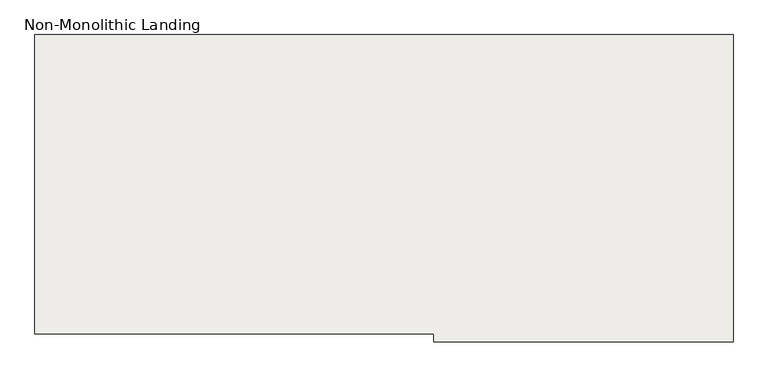
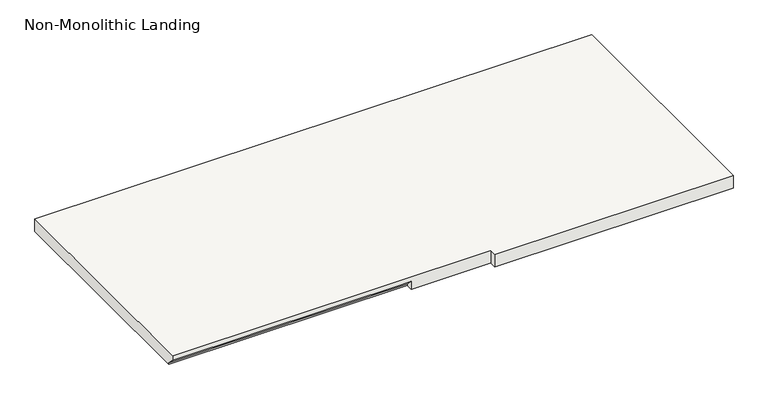
"""IFC4 building model written with IfcOpenShell, lengths in millimetres: slab geometry, Non-Monolithic Landing."""

from ifc_helpers import new_model, si_unit, origin, place, context, project, spatial, faceted_brep, source, transform, mapped, element, save


def non_monolithic_landing_da8bd63b(model_context):
    return source(origin(), model_context, "Body", "Brep", [
        faceted_brep([(-3617.4415084, 23194.7216096, 48752.9005799), (-3617.4415084, 23220.1216096, 48727.5005799), (-2703.0415084, 23220.1216096, 48727.5005799), (-2703.0415084, 23194.7216096, 48752.9005799), (-2398.2415084, 23194.7216096, 48771.9505799), (-2398.2415084, 23169.3216096, 48771.9505799), (-1483.8415084, 23169.3216096, 48771.9505799), (-1483.8415084, 23194.7216096, 48771.9505799), (-1483.8415084, 24109.1216096, 48771.9505799), (-3617.4415084, 24109.1216096, 48771.9505799), (-3617.4415084, 23194.7216096, 48771.9505799), (-2703.0415084, 23220.1216096, 48721.1505799), (-3617.4415084, 23220.1216096, 48721.1505799), (-3617.4415084, 24109.1216096, 48721.1505799), (-1483.8415084, 24109.1216096, 48721.1505799), (-1483.8415084, 23194.7216096, 48721.1505799), (-1483.8415084, 23169.3216096, 48721.1505799), (-2398.2415084, 23169.3216096, 48721.1505799), (-2398.2415084, 23194.7216096, 48721.1505799), (-2703.0415084, 23194.7216096, 48721.1505799)], [[[0, 1, 2, 3]], [[4, 5, 6, 7, 8, 9, 10]], [[11, 12, 13, 14, 15, 16, 17, 18, 19]], [[12, 11, 2, 1]], [[11, 19, 3, 2]], [[4, 10, 0, 3, 19, 18]], [[5, 4, 18, 17]], [[6, 5, 17, 16]], [[7, 6, 16, 15]], [[8, 7, 15, 14]], [[9, 8, 14, 13]], [[10, 9, 13, 12, 1, 0]]]),
    ])


if __name__ == "__main__":
    model = new_model("IFC4")
    model_context = context("Model", 3, world=origin())
    ifc_project = project(units=[si_unit("LENGTHUNIT", "METRE", prefix="MILLI")], contexts=[model_context])
    site = spatial("IfcSite", under=ifc_project)
    building = spatial("IfcBuilding", under=site)
    placement = place(None, origin())
    non_monolithic_landing_shape = non_monolithic_landing_da8bd63b(model_context)
    element("IfcSlab", 1, ObjectType="Non-Monolithic Landing", at=placement, inside=building, context=model_context, shape_type="MappedRepresentation", body=[
        mapped(non_monolithic_landing_shape, transform((0.0, 0.0, 0.0), x_axis=(1.0, 0.0, 0.0), y_axis=(0.0, 1.0, 0.0), z_axis=(0.0, 0.0, 1.0))),
    ])
    save(model, "model.ifc")
